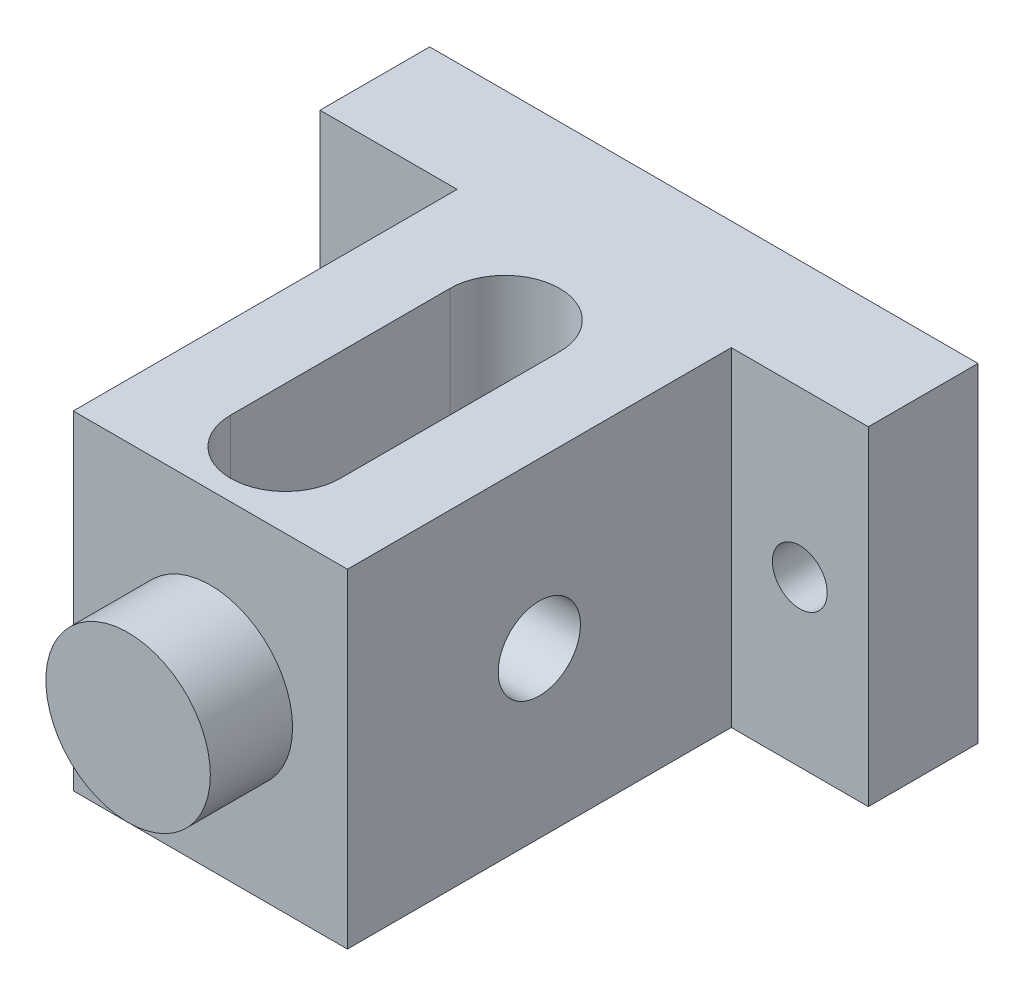
ISO-10303-21;
HEADER;
FILE_DESCRIPTION(('STEP AP214'),'2;1');
FILE_NAME('part.step','',(''),(''),'','','');
FILE_SCHEMA(('AUTOMOTIVE_DESIGN { 1 0 10303 214 1 1 1 1 }'));
ENDSEC;
DATA;
#1=APPLICATION_CONTEXT('core data for automotive mechanical design processes');
#2=APPLICATION_PROTOCOL_DEFINITION('international standard','automotive_design',2000,#1);
#3=PRODUCT_CONTEXT('',#1,'mechanical');
#4=PRODUCT('Part','Part','',(#3));
#5=PRODUCT_RELATED_PRODUCT_CATEGORY('part','',(#4));
#6=PRODUCT_DEFINITION_FORMATION('','',#4);
#7=PRODUCT_DEFINITION_CONTEXT('part definition',#1,'design');
#8=PRODUCT_DEFINITION('design','',#6,#7);
#9=PRODUCT_DEFINITION_SHAPE('','',#8);
#10=(LENGTH_UNIT() NAMED_UNIT(*) SI_UNIT(.MILLI.,.METRE.));
#11=(NAMED_UNIT(*) PLANE_ANGLE_UNIT() SI_UNIT($,.RADIAN.));
#12=(NAMED_UNIT(*) SI_UNIT($,.STERADIAN.) SOLID_ANGLE_UNIT());
#13=UNCERTAINTY_MEASURE_WITH_UNIT(LENGTH_MEASURE(1.E-05),#10,'distance_accuracy_value','');
#14=(GEOMETRIC_REPRESENTATION_CONTEXT(3) GLOBAL_UNCERTAINTY_ASSIGNED_CONTEXT((#13)) GLOBAL_UNIT_ASSIGNED_CONTEXT((#10,
#11,#12)) REPRESENTATION_CONTEXT('',''));
#15=CARTESIAN_POINT('',(0.,0.,0.));
#16=DIRECTION('',(0.,0.,1.));
#17=DIRECTION('',(1.,0.,0.));
#18=AXIS2_PLACEMENT_3D('',#15,#16,#17);
#19=CARTESIAN_POINT('',(0.,0.,20.));
#20=DIRECTION('',(0.,0.,1.));
#21=DIRECTION('',(1.,0.,0.));
#22=AXIS2_PLACEMENT_3D('',#19,#20,#21);
#23=PLANE('',#22);
#24=CARTESIAN_POINT('',(87.5,30.,20.));
#25=DIRECTION('',(0.,0.,1.));
#26=DIRECTION('',(1.,0.,0.));
#27=AXIS2_PLACEMENT_3D('',#24,#25,#26);
#28=CIRCLE('',#27,4.99999999999999);
#29=CARTESIAN_POINT('',(92.5,30.,20.));
#30=VERTEX_POINT('',#29);
#31=EDGE_CURVE('E252',#30,#30,#28,.T.);
#32=ORIENTED_EDGE('',*,*,#31,.F.);
#33=EDGE_LOOP('',(#32));
#34=FACE_BOUND('',#33,.T.);
#35=DIRECTION('',(-1.,0.,0.));
#36=VECTOR('',#35,1.);
#37=CARTESIAN_POINT('',(100.,60.,20.));
#38=LINE('',#37,#36);
#39=CARTESIAN_POINT('',(100.,60.,20.));
#40=VERTEX_POINT('',#39);
#41=CARTESIAN_POINT('',(75.,60.,20.));
#42=VERTEX_POINT('',#41);
#43=EDGE_CURVE('E211',#40,#42,#38,.T.);
#44=ORIENTED_EDGE('',*,*,#43,.T.);
#45=DIRECTION('',(0.,-1.,0.));
#46=VECTOR('',#45,1.);
#47=CARTESIAN_POINT('',(75.,60.,20.));
#48=LINE('',#47,#46);
#49=CARTESIAN_POINT('',(75.,0.,20.));
#50=VERTEX_POINT('',#49);
#51=EDGE_CURVE('E187',#42,#50,#48,.T.);
#52=ORIENTED_EDGE('',*,*,#51,.T.);
#53=DIRECTION('',(1.,0.,0.));
#54=VECTOR('',#53,1.);
#55=CARTESIAN_POINT('',(0.,0.,20.));
#56=LINE('',#55,#54);
#57=CARTESIAN_POINT('',(100.,0.,20.));
#58=VERTEX_POINT('',#57);
#59=EDGE_CURVE('E207',#50,#58,#56,.T.);
#60=ORIENTED_EDGE('',*,*,#59,.T.);
#61=DIRECTION('',(0.,1.,0.));
#62=VECTOR('',#61,1.);
#63=CARTESIAN_POINT('',(100.,0.,20.));
#64=LINE('',#63,#62);
#65=EDGE_CURVE('E212',#58,#40,#64,.T.);
#66=ORIENTED_EDGE('',*,*,#65,.T.);
#67=EDGE_LOOP('',(#44,#52,#60,#66));
#68=FACE_BOUND('',#67,.T.);
#69=ADVANCED_FACE('F44',(#34,#68),#23,.T.);
#70=CARTESIAN_POINT('',(0.,60.,20.));
#71=DIRECTION('',(1.,0.,0.));
#72=DIRECTION('',(0.,0.,-1.));
#73=AXIS2_PLACEMENT_3D('',#70,#71,#72);
#74=PLANE('',#73);
#75=DIRECTION('',(0.,-1.,0.));
#76=VECTOR('',#75,1.);
#77=CARTESIAN_POINT('',(0.,60.,0.));
#78=LINE('',#77,#76);
#79=CARTESIAN_POINT('',(0.,60.,0.));
#80=VERTEX_POINT('',#79);
#81=CARTESIAN_POINT('',(0.,0.,0.));
#82=VERTEX_POINT('',#81);
#83=EDGE_CURVE('E198',#80,#82,#78,.T.);
#84=ORIENTED_EDGE('',*,*,#83,.T.);
#85=DIRECTION('',(0.,0.,-1.));
#86=VECTOR('',#85,1.);
#87=CARTESIAN_POINT('',(0.,0.,20.));
#88=LINE('',#87,#86);
#89=CARTESIAN_POINT('',(0.,0.,20.));
#90=VERTEX_POINT('',#89);
#91=EDGE_CURVE('E53',#90,#82,#88,.T.);
#92=ORIENTED_EDGE('',*,*,#91,.F.);
#93=DIRECTION('',(0.,-1.,0.));
#94=VECTOR('',#93,1.);
#95=CARTESIAN_POINT('',(0.,60.,20.));
#96=LINE('',#95,#94);
#97=CARTESIAN_POINT('',(0.,60.,20.));
#98=VERTEX_POINT('',#97);
#99=EDGE_CURVE('E203',#98,#90,#96,.T.);
#100=ORIENTED_EDGE('',*,*,#99,.F.);
#101=DIRECTION('',(0.,0.,-1.));
#102=VECTOR('',#101,1.);
#103=CARTESIAN_POINT('',(0.,60.,20.));
#104=LINE('',#103,#102);
#105=EDGE_CURVE('E220',#98,#80,#104,.T.);
#106=ORIENTED_EDGE('',*,*,#105,.T.);
#107=EDGE_LOOP('',(#84,#92,#100,#106));
#108=FACE_BOUND('',#107,.T.);
#109=ADVANCED_FACE('F50',(#108),#74,.F.);
#110=CARTESIAN_POINT('',(0.,0.,20.));
#111=DIRECTION('',(0.,1.,0.));
#112=DIRECTION('',(0.,0.,1.));
#113=AXIS2_PLACEMENT_3D('',#110,#111,#112);
#114=PLANE('',#113);
#115=DIRECTION('',(0.,0.,-1.));
#116=VECTOR('',#115,1.);
#117=CARTESIAN_POINT('',(40.,0.,76.2972872501739));
#118=LINE('',#117,#116);
#119=CARTESIAN_POINT('',(40.,0.,76.2972872501739));
#120=VERTEX_POINT('',#119);
#121=CARTESIAN_POINT('',(40.,0.,36.2972872501739));
#122=VERTEX_POINT('',#121);
#123=EDGE_CURVE('E168',#120,#122,#118,.T.);
#124=ORIENTED_EDGE('',*,*,#123,.F.);
#125=CARTESIAN_POINT('',(50.,0.,76.2972872501739));
#126=DIRECTION('',(0.,-1.,0.));
#127=DIRECTION('',(0.,0.,-1.));
#128=AXIS2_PLACEMENT_3D('',#125,#126,#127);
#129=CIRCLE('',#128,10.);
#130=CARTESIAN_POINT('',(60.,0.,76.2972872501739));
#131=VERTEX_POINT('',#130);
#132=EDGE_CURVE('E65',#131,#120,#129,.T.);
#133=ORIENTED_EDGE('',*,*,#132,.F.);
#134=DIRECTION('',(0.,0.,1.));
#135=VECTOR('',#134,1.);
#136=CARTESIAN_POINT('',(60.,0.,36.2972872501739));
#137=LINE('',#136,#135);
#138=CARTESIAN_POINT('',(60.,0.,36.2972872501739));
#139=VERTEX_POINT('',#138);
#140=EDGE_CURVE('E152',#139,#131,#137,.T.);
#141=ORIENTED_EDGE('',*,*,#140,.F.);
#142=CARTESIAN_POINT('',(50.,0.,36.2972872501739));
#143=DIRECTION('',(0.,-1.,0.));
#144=DIRECTION('',(0.,0.,-1.));
#145=AXIS2_PLACEMENT_3D('',#142,#143,#144);
#146=CIRCLE('',#145,10.);
#147=EDGE_CURVE('E160',#122,#139,#146,.T.);
#148=ORIENTED_EDGE('',*,*,#147,.F.);
#149=EDGE_LOOP('',(#124,#133,#141,#148));
#150=FACE_BOUND('',#149,.T.);
#151=DIRECTION('',(1.,0.,0.));
#152=VECTOR('',#151,1.);
#153=CARTESIAN_POINT('',(0.,0.,0.));
#154=LINE('',#153,#152);
#155=CARTESIAN_POINT('',(100.,0.,0.));
#156=VERTEX_POINT('',#155);
#157=EDGE_CURVE('E219',#82,#156,#154,.T.);
#158=ORIENTED_EDGE('',*,*,#157,.T.);
#159=DIRECTION('',(0.,0.,-1.));
#160=VECTOR('',#159,1.);
#161=CARTESIAN_POINT('',(100.,0.,20.));
#162=LINE('',#161,#160);
#163=EDGE_CURVE('E229',#58,#156,#162,.T.);
#164=ORIENTED_EDGE('',*,*,#163,.F.);
#165=ORIENTED_EDGE('',*,*,#59,.F.);
#166=DIRECTION('',(0.,0.,1.));
#167=VECTOR('',#166,1.);
#168=CARTESIAN_POINT('',(75.,0.,90.));
#169=LINE('',#168,#167);
#170=CARTESIAN_POINT('',(75.,0.,90.));
#171=VERTEX_POINT('',#170);
#172=EDGE_CURVE('E173',#50,#171,#169,.T.);
#173=ORIENTED_EDGE('',*,*,#172,.T.);
#174=DIRECTION('',(-1.,0.,0.));
#175=VECTOR('',#174,1.);
#176=CARTESIAN_POINT('',(25.,0.,90.));
#177=LINE('',#176,#175);
#178=CARTESIAN_POINT('',(25.,0.,90.));
#179=VERTEX_POINT('',#178);
#180=EDGE_CURVE('E186',#171,#179,#177,.T.);
#181=ORIENTED_EDGE('',*,*,#180,.T.);
#182=DIRECTION('',(0.,0.,-1.));
#183=VECTOR('',#182,1.);
#184=CARTESIAN_POINT('',(25.,0.,20.));
#185=LINE('',#184,#183);
#186=CARTESIAN_POINT('',(25.,0.,20.));
#187=VERTEX_POINT('',#186);
#188=EDGE_CURVE('E181',#179,#187,#185,.T.);
#189=ORIENTED_EDGE('',*,*,#188,.T.);
#190=EDGE_CURVE('E206',#90,#187,#56,.T.);
#191=ORIENTED_EDGE('',*,*,#190,.F.);
#192=ORIENTED_EDGE('',*,*,#91,.T.);
#193=EDGE_LOOP('',(#158,#164,#165,#173,#181,#189,#191,#192));
#194=FACE_BOUND('',#193,.T.);
#195=ADVANCED_FACE('F281',(#150,#194),#114,.F.);
#196=CARTESIAN_POINT('',(100.,0.,20.));
#197=DIRECTION('',(-1.,0.,0.));
#198=DIRECTION('',(0.,0.,1.));
#199=AXIS2_PLACEMENT_3D('',#196,#197,#198);
#200=PLANE('',#199);
#201=DIRECTION('',(0.,1.,0.));
#202=VECTOR('',#201,1.);
#203=CARTESIAN_POINT('',(100.,0.,0.));
#204=LINE('',#203,#202);
#205=CARTESIAN_POINT('',(100.,60.,0.));
#206=VERTEX_POINT('',#205);
#207=EDGE_CURVE('E225',#156,#206,#204,.T.);
#208=ORIENTED_EDGE('',*,*,#207,.T.);
#209=DIRECTION('',(0.,0.,-1.));
#210=VECTOR('',#209,1.);
#211=CARTESIAN_POINT('',(100.,60.,20.));
#212=LINE('',#211,#210);
#213=EDGE_CURVE('E227',#40,#206,#212,.T.);
#214=ORIENTED_EDGE('',*,*,#213,.F.);
#215=ORIENTED_EDGE('',*,*,#65,.F.);
#216=ORIENTED_EDGE('',*,*,#163,.T.);
#217=EDGE_LOOP('',(#208,#214,#215,#216));
#218=FACE_BOUND('',#217,.T.);
#219=ADVANCED_FACE('F299',(#218),#200,.F.);
#220=CARTESIAN_POINT('',(100.,60.,20.));
#221=DIRECTION('',(0.,-1.,0.));
#222=DIRECTION('',(0.,0.,-1.));
#223=AXIS2_PLACEMENT_3D('',#220,#221,#222);
#224=PLANE('',#223);
#225=DIRECTION('',(0.,0.,1.));
#226=VECTOR('',#225,1.);
#227=CARTESIAN_POINT('',(60.,60.,36.2972872501739));
#228=LINE('',#227,#226);
#229=CARTESIAN_POINT('',(60.,60.,36.2972872501739));
#230=VERTEX_POINT('',#229);
#231=CARTESIAN_POINT('',(60.,60.,76.2972872501739));
#232=VERTEX_POINT('',#231);
#233=EDGE_CURVE('E144',#230,#232,#228,.T.);
#234=ORIENTED_EDGE('',*,*,#233,.T.);
#235=CARTESIAN_POINT('',(50.,60.,76.2972872501739));
#236=DIRECTION('',(0.,-1.,0.));
#237=DIRECTION('',(0.,0.,-1.));
#238=AXIS2_PLACEMENT_3D('',#235,#236,#237);
#239=CIRCLE('',#238,10.);
#240=CARTESIAN_POINT('',(40.,60.,76.2972872501739));
#241=VERTEX_POINT('',#240);
#242=EDGE_CURVE('E138',#232,#241,#239,.T.);
#243=ORIENTED_EDGE('',*,*,#242,.T.);
#244=DIRECTION('',(0.,0.,-1.));
#245=VECTOR('',#244,1.);
#246=CARTESIAN_POINT('',(40.,60.,76.2972872501739));
#247=LINE('',#246,#245);
#248=CARTESIAN_POINT('',(40.,60.,36.2972872501739));
#249=VERTEX_POINT('',#248);
#250=EDGE_CURVE('E150',#241,#249,#247,.T.);
#251=ORIENTED_EDGE('',*,*,#250,.T.);
#252=CARTESIAN_POINT('',(50.,60.,36.2972872501739));
#253=DIRECTION('',(0.,-1.,0.));
#254=DIRECTION('',(0.,0.,-1.));
#255=AXIS2_PLACEMENT_3D('',#252,#253,#254);
#256=CIRCLE('',#255,10.);
#257=EDGE_CURVE('E69',#249,#230,#256,.T.);
#258=ORIENTED_EDGE('',*,*,#257,.T.);
#259=EDGE_LOOP('',(#234,#243,#251,#258));
#260=FACE_BOUND('',#259,.T.);
#261=DIRECTION('',(-1.,0.,0.));
#262=VECTOR('',#261,1.);
#263=CARTESIAN_POINT('',(100.,60.,0.));
#264=LINE('',#263,#262);
#265=EDGE_CURVE('E210',#206,#80,#264,.T.);
#266=ORIENTED_EDGE('',*,*,#265,.T.);
#267=ORIENTED_EDGE('',*,*,#105,.F.);
#268=CARTESIAN_POINT('',(25.,60.,20.));
#269=VERTEX_POINT('',#268);
#270=EDGE_CURVE('E214',#269,#98,#38,.T.);
#271=ORIENTED_EDGE('',*,*,#270,.F.);
#272=DIRECTION('',(0.,0.,-1.));
#273=VECTOR('',#272,1.);
#274=CARTESIAN_POINT('',(25.,60.,20.));
#275=LINE('',#274,#273);
#276=CARTESIAN_POINT('',(25.,60.,90.));
#277=VERTEX_POINT('',#276);
#278=EDGE_CURVE('E183',#277,#269,#275,.T.);
#279=ORIENTED_EDGE('',*,*,#278,.F.);
#280=DIRECTION('',(-1.,0.,0.));
#281=VECTOR('',#280,1.);
#282=CARTESIAN_POINT('',(25.,60.,90.));
#283=LINE('',#282,#281);
#284=CARTESIAN_POINT('',(75.,60.,90.));
#285=VERTEX_POINT('',#284);
#286=EDGE_CURVE('E179',#285,#277,#283,.T.);
#287=ORIENTED_EDGE('',*,*,#286,.F.);
#288=DIRECTION('',(0.,0.,1.));
#289=VECTOR('',#288,1.);
#290=CARTESIAN_POINT('',(75.,60.,90.));
#291=LINE('',#290,#289);
#292=EDGE_CURVE('E180',#42,#285,#291,.T.);
#293=ORIENTED_EDGE('',*,*,#292,.F.);
#294=ORIENTED_EDGE('',*,*,#43,.F.);
#295=ORIENTED_EDGE('',*,*,#213,.T.);
#296=EDGE_LOOP('',(#266,#267,#271,#279,#287,#293,#294,#295));
#297=FACE_BOUND('',#296,.T.);
#298=ADVANCED_FACE('F153',(#260,#297),#224,.F.);
#299=CARTESIAN_POINT('',(13.01615859241,30.,20.));
#300=DIRECTION('',(0.,0.,1.));
#301=DIRECTION('',(1.,0.,0.));
#302=AXIS2_PLACEMENT_3D('',#299,#300,#301);
#303=CIRCLE('',#302,5.);
#304=CARTESIAN_POINT('',(18.01615859241,30.,20.));
#305=VERTEX_POINT('',#304);
#306=EDGE_CURVE('E156',#305,#305,#303,.T.);
#307=ORIENTED_EDGE('',*,*,#306,.F.);
#308=EDGE_LOOP('',(#307));
#309=FACE_BOUND('',#308,.T.);
#310=DIRECTION('',(0.,-1.,0.));
#311=VECTOR('',#310,1.);
#312=CARTESIAN_POINT('',(25.,60.,20.));
#313=LINE('',#312,#311);
#314=EDGE_CURVE('E191',#269,#187,#313,.T.);
#315=ORIENTED_EDGE('',*,*,#314,.F.);
#316=ORIENTED_EDGE('',*,*,#270,.T.);
#317=ORIENTED_EDGE('',*,*,#99,.T.);
#318=ORIENTED_EDGE('',*,*,#190,.T.);
#319=EDGE_LOOP('',(#315,#316,#317,#318));
#320=FACE_BOUND('',#319,.T.);
#321=ADVANCED_FACE('F267',(#309,#320),#23,.T.);
#322=CARTESIAN_POINT('',(0.,0.,0.));
#323=DIRECTION('',(0.,0.,1.));
#324=DIRECTION('',(1.,0.,0.));
#325=AXIS2_PLACEMENT_3D('',#322,#323,#324);
#326=PLANE('',#325);
#327=CARTESIAN_POINT('',(87.5,30.,0.));
#328=DIRECTION('',(0.,0.,1.));
#329=DIRECTION('',(1.,0.,0.));
#330=AXIS2_PLACEMENT_3D('',#327,#328,#329);
#331=CIRCLE('',#330,4.99999999999999);
#332=CARTESIAN_POINT('',(92.5,30.,0.));
#333=VERTEX_POINT('',#332);
#334=EDGE_CURVE('E170',#333,#333,#331,.T.);
#335=ORIENTED_EDGE('',*,*,#334,.T.);
#336=EDGE_LOOP('',(#335));
#337=FACE_BOUND('',#336,.T.);
#338=CARTESIAN_POINT('',(13.01615859241,30.,0.));
#339=DIRECTION('',(0.,0.,1.));
#340=DIRECTION('',(1.,0.,0.));
#341=AXIS2_PLACEMENT_3D('',#338,#339,#340);
#342=CIRCLE('',#341,5.);
#343=CARTESIAN_POINT('',(18.01615859241,30.,0.));
#344=VERTEX_POINT('',#343);
#345=EDGE_CURVE('E239',#344,#344,#342,.T.);
#346=ORIENTED_EDGE('',*,*,#345,.T.);
#347=EDGE_LOOP('',(#346));
#348=FACE_BOUND('',#347,.T.);
#349=ORIENTED_EDGE('',*,*,#83,.F.);
#350=ORIENTED_EDGE('',*,*,#265,.F.);
#351=ORIENTED_EDGE('',*,*,#207,.F.);
#352=ORIENTED_EDGE('',*,*,#157,.F.);
#353=EDGE_LOOP('',(#349,#350,#351,#352));
#354=FACE_BOUND('',#353,.T.);
#355=ADVANCED_FACE('F257',(#337,#348,#354),#326,.F.);
#356=CARTESIAN_POINT('',(25.,60.,20.));
#357=DIRECTION('',(-1.,0.,0.));
#358=DIRECTION('',(0.,0.,1.));
#359=AXIS2_PLACEMENT_3D('',#356,#357,#358);
#360=PLANE('',#359);
#361=CARTESIAN_POINT('',(25.,30.,55.));
#362=DIRECTION('',(-1.,0.,0.));
#363=DIRECTION('',(0.,0.,1.));
#364=AXIS2_PLACEMENT_3D('',#361,#362,#363);
#365=CIRCLE('',#364,7.5);
#366=CARTESIAN_POINT('',(25.,30.,62.5));
#367=VERTEX_POINT('',#366);
#368=EDGE_CURVE('E246',#367,#367,#365,.T.);
#369=ORIENTED_EDGE('',*,*,#368,.F.);
#370=EDGE_LOOP('',(#369));
#371=FACE_BOUND('',#370,.T.);
#372=ORIENTED_EDGE('',*,*,#188,.F.);
#373=DIRECTION('',(0.,-1.,0.));
#374=VECTOR('',#373,1.);
#375=CARTESIAN_POINT('',(25.,60.,90.));
#376=LINE('',#375,#374);
#377=EDGE_CURVE('E200',#277,#179,#376,.T.);
#378=ORIENTED_EDGE('',*,*,#377,.F.);
#379=ORIENTED_EDGE('',*,*,#278,.T.);
#380=ORIENTED_EDGE('',*,*,#314,.T.);
#381=EDGE_LOOP('',(#372,#378,#379,#380));
#382=FACE_BOUND('',#381,.T.);
#383=ADVANCED_FACE('F287',(#371,#382),#360,.T.);
#384=CARTESIAN_POINT('',(25.,60.,90.));
#385=DIRECTION('',(0.,0.,1.));
#386=DIRECTION('',(1.,0.,0.));
#387=AXIS2_PLACEMENT_3D('',#384,#385,#386);
#388=PLANE('',#387);
#389=CARTESIAN_POINT('',(50.,30.,90.));
#390=DIRECTION('',(0.,0.,1.));
#391=DIRECTION('',(1.,0.,0.));
#392=AXIS2_PLACEMENT_3D('',#389,#390,#391);
#393=CIRCLE('',#392,15.);
#394=CARTESIAN_POINT('',(65.,30.,90.));
#395=VERTEX_POINT('',#394);
#396=EDGE_CURVE('E11',#395,#395,#393,.T.);
#397=ORIENTED_EDGE('',*,*,#396,.F.);
#398=EDGE_LOOP('',(#397));
#399=FACE_BOUND('',#398,.T.);
#400=ORIENTED_EDGE('',*,*,#180,.F.);
#401=DIRECTION('',(0.,-1.,0.));
#402=VECTOR('',#401,1.);
#403=CARTESIAN_POINT('',(75.,60.,90.));
#404=LINE('',#403,#402);
#405=EDGE_CURVE('E197',#285,#171,#404,.T.);
#406=ORIENTED_EDGE('',*,*,#405,.F.);
#407=ORIENTED_EDGE('',*,*,#286,.T.);
#408=ORIENTED_EDGE('',*,*,#377,.T.);
#409=EDGE_LOOP('',(#400,#406,#407,#408));
#410=FACE_BOUND('',#409,.T.);
#411=ADVANCED_FACE('F288',(#399,#410),#388,.T.);
#412=CARTESIAN_POINT('',(75.,60.,90.));
#413=DIRECTION('',(1.,0.,0.));
#414=DIRECTION('',(0.,0.,-1.));
#415=AXIS2_PLACEMENT_3D('',#412,#413,#414);
#416=PLANE('',#415);
#417=CARTESIAN_POINT('',(75.,30.,55.));
#418=DIRECTION('',(1.,0.,0.));
#419=DIRECTION('',(0.,0.,-1.));
#420=AXIS2_PLACEMENT_3D('',#417,#418,#419);
#421=CIRCLE('',#420,7.5);
#422=CARTESIAN_POINT('',(75.,30.,47.5));
#423=VERTEX_POINT('',#422);
#424=EDGE_CURVE('E236',#423,#423,#421,.T.);
#425=ORIENTED_EDGE('',*,*,#424,.F.);
#426=EDGE_LOOP('',(#425));
#427=FACE_BOUND('',#426,.T.);
#428=ORIENTED_EDGE('',*,*,#172,.F.);
#429=ORIENTED_EDGE('',*,*,#51,.F.);
#430=ORIENTED_EDGE('',*,*,#292,.T.);
#431=ORIENTED_EDGE('',*,*,#405,.T.);
#432=EDGE_LOOP('',(#428,#429,#430,#431));
#433=FACE_BOUND('',#432,.T.);
#434=ADVANCED_FACE('F292',(#427,#433),#416,.T.);
#435=CARTESIAN_POINT('',(50.,60.,76.2972872501739));
#436=DIRECTION('',(0.,-1.,0.));
#437=DIRECTION('',(0.,0.,-1.));
#438=AXIS2_PLACEMENT_3D('',#435,#436,#437);
#439=CYLINDRICAL_SURFACE('',#438,10.);
#440=ORIENTED_EDGE('',*,*,#132,.T.);
#441=DIRECTION('',(0.,-1.,0.));
#442=VECTOR('',#441,1.);
#443=CARTESIAN_POINT('',(40.,60.,76.2972872501739));
#444=LINE('',#443,#442);
#445=EDGE_CURVE('E132',#241,#120,#444,.T.);
#446=ORIENTED_EDGE('',*,*,#445,.F.);
#447=ORIENTED_EDGE('',*,*,#242,.F.);
#448=DIRECTION('',(0.,-1.,0.));
#449=VECTOR('',#448,1.);
#450=CARTESIAN_POINT('',(60.,60.,76.2972872501739));
#451=LINE('',#450,#449);
#452=EDGE_CURVE('E171',#232,#131,#451,.T.);
#453=ORIENTED_EDGE('',*,*,#452,.T.);
#454=EDGE_LOOP('',(#440,#446,#447,#453));
#455=FACE_BOUND('',#454,.T.);
#456=ADVANCED_FACE('F137',(#455),#439,.F.);
#457=CARTESIAN_POINT('',(60.,60.,36.2972872501739));
#458=DIRECTION('',(1.,0.,0.));
#459=DIRECTION('',(0.,0.,-1.));
#460=AXIS2_PLACEMENT_3D('',#457,#458,#459);
#461=PLANE('',#460);
#462=CARTESIAN_POINT('',(60.,30.,55.));
#463=DIRECTION('',(1.,0.,0.));
#464=DIRECTION('',(0.,0.,-1.));
#465=AXIS2_PLACEMENT_3D('',#462,#463,#464);
#466=CIRCLE('',#465,7.5);
#467=CARTESIAN_POINT('',(60.,30.,47.5));
#468=VERTEX_POINT('',#467);
#469=EDGE_CURVE('E234',#468,#468,#466,.T.);
#470=ORIENTED_EDGE('',*,*,#469,.T.);
#471=EDGE_LOOP('',(#470));
#472=FACE_BOUND('',#471,.T.);
#473=ORIENTED_EDGE('',*,*,#140,.T.);
#474=ORIENTED_EDGE('',*,*,#452,.F.);
#475=ORIENTED_EDGE('',*,*,#233,.F.);
#476=DIRECTION('',(0.,-1.,0.));
#477=VECTOR('',#476,1.);
#478=CARTESIAN_POINT('',(60.,60.,36.2972872501739));
#479=LINE('',#478,#477);
#480=EDGE_CURVE('E172',#230,#139,#479,.T.);
#481=ORIENTED_EDGE('',*,*,#480,.T.);
#482=EDGE_LOOP('',(#473,#474,#475,#481));
#483=FACE_BOUND('',#482,.T.);
#484=ADVANCED_FACE('F328',(#472,#483),#461,.F.);
#485=CARTESIAN_POINT('',(50.,60.,36.2972872501739));
#486=DIRECTION('',(0.,-1.,0.));
#487=DIRECTION('',(0.,0.,-1.));
#488=AXIS2_PLACEMENT_3D('',#485,#486,#487);
#489=CYLINDRICAL_SURFACE('',#488,10.);
#490=ORIENTED_EDGE('',*,*,#147,.T.);
#491=ORIENTED_EDGE('',*,*,#480,.F.);
#492=ORIENTED_EDGE('',*,*,#257,.F.);
#493=DIRECTION('',(0.,-1.,0.));
#494=VECTOR('',#493,1.);
#495=CARTESIAN_POINT('',(40.,60.,36.2972872501739));
#496=LINE('',#495,#494);
#497=EDGE_CURVE('E141',#249,#122,#496,.T.);
#498=ORIENTED_EDGE('',*,*,#497,.T.);
#499=EDGE_LOOP('',(#490,#491,#492,#498));
#500=FACE_BOUND('',#499,.T.);
#501=ADVANCED_FACE('F327',(#500),#489,.F.);
#502=CARTESIAN_POINT('',(40.,60.,76.2972872501739));
#503=DIRECTION('',(-1.,0.,0.));
#504=DIRECTION('',(0.,0.,1.));
#505=AXIS2_PLACEMENT_3D('',#502,#503,#504);
#506=PLANE('',#505);
#507=CARTESIAN_POINT('',(40.,30.,55.));
#508=DIRECTION('',(-1.,0.,0.));
#509=DIRECTION('',(0.,0.,1.));
#510=AXIS2_PLACEMENT_3D('',#507,#508,#509);
#511=CIRCLE('',#510,7.5);
#512=CARTESIAN_POINT('',(40.,30.,62.5));
#513=VERTEX_POINT('',#512);
#514=EDGE_CURVE('E47',#513,#513,#511,.T.);
#515=ORIENTED_EDGE('',*,*,#514,.T.);
#516=EDGE_LOOP('',(#515));
#517=FACE_BOUND('',#516,.T.);
#518=ORIENTED_EDGE('',*,*,#123,.T.);
#519=ORIENTED_EDGE('',*,*,#497,.F.);
#520=ORIENTED_EDGE('',*,*,#250,.F.);
#521=ORIENTED_EDGE('',*,*,#445,.T.);
#522=EDGE_LOOP('',(#518,#519,#520,#521));
#523=FACE_BOUND('',#522,.T.);
#524=ADVANCED_FACE('F149',(#517,#523),#506,.F.);
#525=CARTESIAN_POINT('',(13.01615859241,30.,0.));
#526=DIRECTION('',(0.,0.,1.));
#527=DIRECTION('',(1.,0.,0.));
#528=AXIS2_PLACEMENT_3D('',#525,#526,#527);
#529=CYLINDRICAL_SURFACE('',#528,5.);
#530=ORIENTED_EDGE('',*,*,#345,.F.);
#531=EDGE_LOOP('',(#530));
#532=FACE_BOUND('',#531,.T.);
#533=ORIENTED_EDGE('',*,*,#306,.T.);
#534=EDGE_LOOP('',(#533));
#535=FACE_BOUND('',#534,.T.);
#536=ADVANCED_FACE('F256',(#532,#535),#529,.F.);
#537=CARTESIAN_POINT('',(87.5,30.,0.));
#538=DIRECTION('',(0.,0.,1.));
#539=DIRECTION('',(1.,0.,0.));
#540=AXIS2_PLACEMENT_3D('',#537,#538,#539);
#541=CYLINDRICAL_SURFACE('',#540,4.99999999999999);
#542=ORIENTED_EDGE('',*,*,#334,.F.);
#543=EDGE_LOOP('',(#542));
#544=FACE_BOUND('',#543,.T.);
#545=ORIENTED_EDGE('',*,*,#31,.T.);
#546=EDGE_LOOP('',(#545));
#547=FACE_BOUND('',#546,.T.);
#548=ADVANCED_FACE('F265',(#544,#547),#541,.F.);
#549=CARTESIAN_POINT('',(50.,30.,55.));
#550=DIRECTION('',(1.,0.,0.));
#551=DIRECTION('',(0.,0.,-1.));
#552=AXIS2_PLACEMENT_3D('',#549,#550,#551);
#553=CYLINDRICAL_SURFACE('',#552,7.5);
#554=ORIENTED_EDGE('',*,*,#424,.T.);
#555=EDGE_LOOP('',(#554));
#556=FACE_BOUND('',#555,.T.);
#557=ORIENTED_EDGE('',*,*,#469,.F.);
#558=EDGE_LOOP('',(#557));
#559=FACE_BOUND('',#558,.T.);
#560=ADVANCED_FACE('F337',(#556,#559),#553,.F.);
#561=CARTESIAN_POINT('',(50.,30.,55.));
#562=DIRECTION('',(-1.,0.,0.));
#563=DIRECTION('',(0.,0.,1.));
#564=AXIS2_PLACEMENT_3D('',#561,#562,#563);
#565=CYLINDRICAL_SURFACE('',#564,7.5);
#566=ORIENTED_EDGE('',*,*,#368,.T.);
#567=EDGE_LOOP('',(#566));
#568=FACE_BOUND('',#567,.T.);
#569=ORIENTED_EDGE('',*,*,#514,.F.);
#570=EDGE_LOOP('',(#569));
#571=FACE_BOUND('',#570,.T.);
#572=ADVANCED_FACE('F338',(#568,#571),#565,.F.);
#573=CARTESIAN_POINT('',(50.,30.,105.));
#574=DIRECTION('',(0.,0.,-1.));
#575=DIRECTION('',(-1.,0.,0.));
#576=AXIS2_PLACEMENT_3D('',#573,#574,#575);
#577=CYLINDRICAL_SURFACE('',#576,15.);
#578=CARTESIAN_POINT('',(50.,30.,105.));
#579=DIRECTION('',(0.,0.,1.));
#580=DIRECTION('',(1.,0.,0.));
#581=AXIS2_PLACEMENT_3D('',#578,#579,#580);
#582=CIRCLE('',#581,15.);
#583=CARTESIAN_POINT('',(65.,30.,105.));
#584=VERTEX_POINT('',#583);
#585=EDGE_CURVE('E351',#584,#584,#582,.T.);
#586=ORIENTED_EDGE('',*,*,#585,.F.);
#587=EDGE_LOOP('',(#586));
#588=FACE_BOUND('',#587,.T.);
#589=ORIENTED_EDGE('',*,*,#396,.T.);
#590=EDGE_LOOP('',(#589));
#591=FACE_BOUND('',#590,.T.);
#592=ADVANCED_FACE('F344',(#588,#591),#577,.T.);
#593=CARTESIAN_POINT('',(50.,30.,105.));
#594=DIRECTION('',(0.,0.,1.));
#595=DIRECTION('',(1.,0.,0.));
#596=AXIS2_PLACEMENT_3D('',#593,#594,#595);
#597=PLANE('',#596);
#598=ORIENTED_EDGE('',*,*,#585,.T.);
#599=EDGE_LOOP('',(#598));
#600=FACE_BOUND('',#599,.T.);
#601=ADVANCED_FACE('F350',(#600),#597,.T.);
#602=CLOSED_SHELL('',(#69,#109,#195,#219,#298,#321,#355,#383,#411,#434,#456,#484,#501,#524,#536,
#548,#560,#572,#592,#601));
#603=MANIFOLD_SOLID_BREP('B2',#602);
#604=ADVANCED_BREP_SHAPE_REPRESENTATION('',(#18,#603),#14);
#605=SHAPE_DEFINITION_REPRESENTATION(#9,#604);
ENDSEC;
END-ISO-10303-21;
